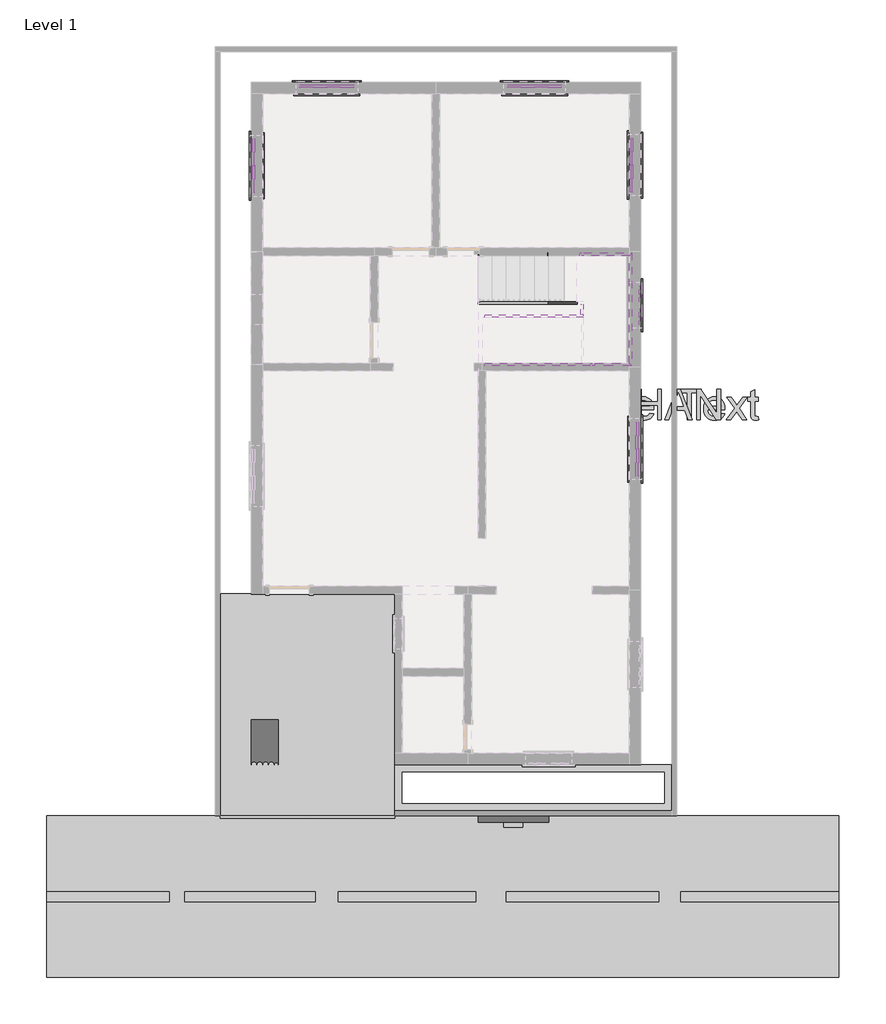
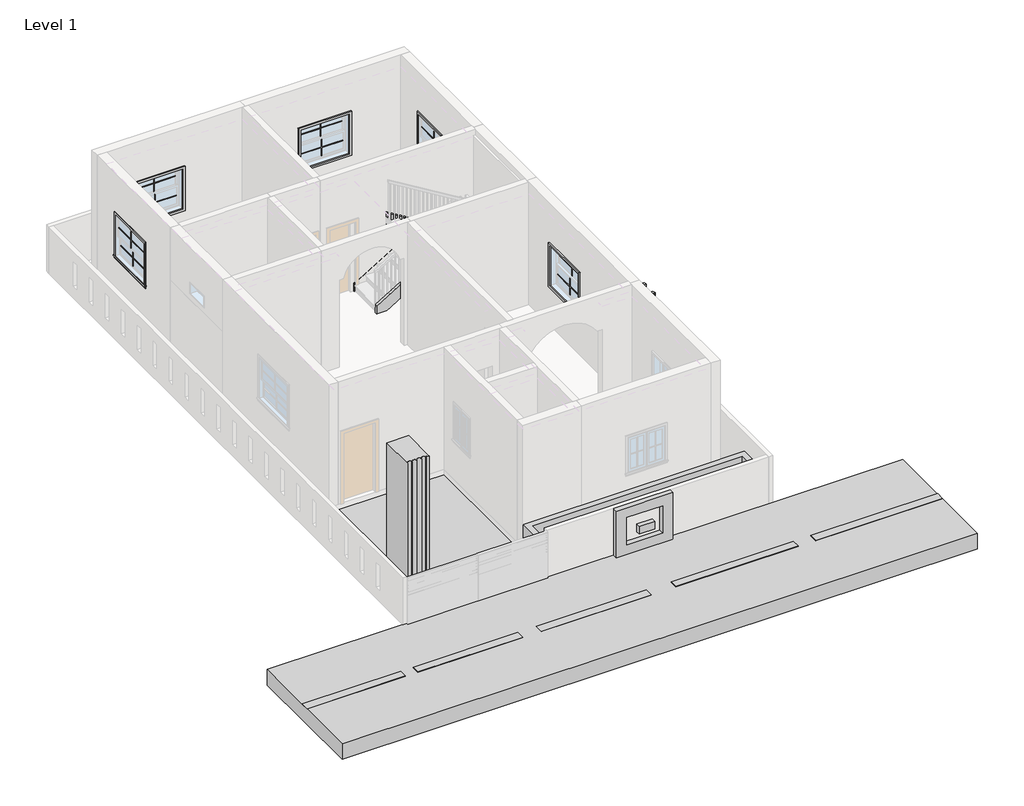
# One storey, part 3 of 3: 32 proxies, 8 members.
"""IFC4 building model written with IfcOpenShell, lengths in millimetres."""

from ifc_helpers import new_model, si_unit, frame, origin, origin_with_axes, place, context, project, spatial, polyline, outline, extrude, faceted_brep, transform, mapped, element, save
from components import generic_models_4629e616, design_design_48f371e7, generic_models_1_generic_models_1_2bf1bac3, generic_models_2_generic_models_2_314bea4d, muntin_pattern_2x2_muntin_pattern_2x2_8b3f23e7, muntin_pattern_2x2_muntin_pattern_2x2_5e52a1c6, muntin_pattern_2x2_muntin_pattern_2x2_d1c6e638, muntin_pattern_2x2_muntin_pattern_2x2_37b95fb2, trim_window_exterior_flat_with_sill_f44f30ad, trim_window_exterior_flat_with_sill_e2e7eb1d, trim_window_exterior_flat_with_sill_84e24481, trim_window_interior_flat_picture_frame_1dce1945, trim_window_interior_flat_picture_frame_a40cb921, trim_window_interior_flat_picture_frame_28d4e5dc

model = new_model("IFC4")

# Units and contexts
model_context = context("Model", 3, world=origin())
ifc_project = project(units=[si_unit("LENGTHUNIT", "METRE", prefix="MILLI")], contexts=[model_context])

# Site, building, storey
site = spatial("IfcSite", under=ifc_project)
building = spatial("IfcBuilding", under=site)
storey = spatial("IfcBuildingStorey", under=building, Name="Level 1", Elevation=0.0)

# Proxies
placement = place(None, origin())
generic_models_shape = generic_models_4629e616(model_context)
element("IfcBuildingElementProxy", 1, Name="Generic Models", at=placement, inside=storey, context=model_context, shape_type="MappedRepresentation", body=[
    mapped(generic_models_shape, transform((0.0, 0.0, 0.0), x_axis=(1.0, 0.0, 0.0), y_axis=(0.0, 1.0, 0.0), z_axis=(0.0, 0.0, 1.0))),
])
element("IfcBuildingElementProxy", 2, Name="24\" Arial", ObjectType="24\" Arial", at=placement, inside=storey, context=model_context, shape_type="SweptSolid", body=[
    extrude(outline(polyline([(66.6240518, 0.0), (66.6240518, 609.1341881), (197.1952963, 609.1341881), (322.1153934, 179.7957113), (347.3968417, 90.1209272), (374.6115771, 187.2314314), (497.1522439, 609.1341881), (628.1696315, 609.1341881), (628.1696315, 0.0), (552.027858, 0.0), (552.027858, 532.9924146), (399.000739, 0.0), (295.9416588, 0.0), (142.7658253, 532.9924146), (142.7658253, 0.0), (66.6240518, 0.0)])), origin_with_axes(), (0.0, 0.0, 1.0), 152.4),
    extrude(outline(polyline([(732.8645701, 223.6664597), (736.9821001, 281.6000137), (749.3346901, 331.5215793), (769.92234, 373.4311566), (798.7450499, 407.3287454), (827.7629475, 428.9945748), (859.7923117, 444.4701672), (894.8331425, 453.7555226), (932.88544, 456.8506411), (974.8926111, 453.0816605), (1012.8751986, 441.7747187), (1046.8332027, 422.9298156), (1076.7666233, 396.5469513), (1101.1976111, 363.5184122), (1118.6483166, 324.7364848), (1129.11874, 280.2011689), (1132.6088811, 229.9124646), (1131.0659692, 189.1554239), (1126.4372334, 152.9899404), (1118.7226738, 121.4160141), (1107.9222904, 94.4336449), (1094.1708556, 71.1273098), (1077.6031418, 50.5814858), (1058.2191491, 32.7961728), (1036.0188774, 17.771371), (1011.8667291, 5.8323929), (986.6271068, -2.6954485), (960.3000104, -7.8121534), (932.88544, -9.5177217), (890.264822, -5.7626831), (851.9290377, 5.5024329), (817.8780871, 24.277626), (788.1119702, 50.5628965), (763.9412327, 83.912101), (746.6764201, 123.8790964), (736.3175326, 170.4638826), (732.8645701, 223.6664597)]), holes=[polyline([(809.0063436, 223.8151741), (811.2091757, 186.882882), (817.8176719, 154.9046384), (828.8318323, 127.8804432), (844.2516568, 105.8102966), (863.0082606, 88.6663145), (884.0327591, 76.420613), (907.3251522, 69.0731921), (932.88544, 66.6240518), (958.3156026, 69.0871341), (981.5150492, 76.4763809), (1002.4837798, 88.7917923), (1021.2217944, 106.0333682), (1036.6416189, 128.3219391), (1047.6557793, 155.7783355), (1054.2642755, 188.4025573), (1056.4671075, 226.1946045), (1054.2503335, 261.9557707), (1047.6000114, 293.0974959), (1036.5161411, 319.6197799), (1020.9987228, 341.5226228), (1002.1909984, 358.6666049), (981.2362097, 370.9123064), (958.1343569, 378.2597273), (932.88544, 380.7088676), (907.3251522, 378.2690219), (884.0327591, 370.949485), (863.0082606, 358.7502568), (844.2516568, 341.6713372), (828.8318323, 319.6662531), (817.8176719, 292.6885313), (811.2091757, 260.7381716), (809.0063436, 223.8151741)])]), origin_with_axes(), (0.0, 0.0, 1.0), 152.4),
    extrude(outline(polyline([(1494.2823053, 0.0), (1494.2823053, 71.8290559), (1471.5011179, 36.2398407), (1443.9053018, 10.8189727), (1411.4948569, -4.4335481), (1374.2697833, -9.5177217), (1349.1370495, -7.677381), (1325.0453165, -2.1563588), (1301.9945843, 7.0453448), (1279.9848529, 19.9277298), (1259.7039264, 36.1050683), (1241.8396089, 55.1916322), (1226.3919004, 77.1874217), (1213.360801, 102.0924366), (1203.0158555, 129.4326498), (1195.6266087, 158.7340342), (1189.7152112, 223.2203165), (1195.1618762, 286.9072589), (1211.501871, 344.4225536), (1223.7522198, 370.0479039), (1238.7166065, 392.4944839), (1256.3950309, 411.7622935), (1276.7874932, 427.8513328), (1299.173658, 440.5385302), (1322.8331898, 449.600814), (1347.7660886, 455.0381843), (1373.9723545, 456.8506411), (1411.2253121, 451.6642264), (1444.165552, 436.1049821), (1472.0866809, 412.25491), (1494.2823053, 382.1960116), (1494.2823053, 609.1341881), (1570.4240788, 609.1341881), (1570.4240788, 0.0), (1494.2823053, 0.0)]), holes=[polyline([(1265.8569847, 223.5177453), (1268.0040489, 186.5947478), (1274.4452414, 154.6443882), (1285.1805623, 127.6666663), (1300.2100114, 105.6615822), (1318.1579808, 88.5826627), (1337.648862, 76.3834344), (1358.6826551, 69.0638975), (1381.2593602, 66.6240518), (1403.9429537, 68.9523617), (1424.8512691, 75.9372912), (1443.9843063, 87.5788404), (1461.3420654, 103.8770094), (1475.7534203, 124.9619231), (1486.0472453, 150.9637067), (1492.2235403, 181.8823602), (1494.2823053, 217.7178837), (1492.1863617, 257.0063696), (1485.8985309, 290.6994761), (1475.4188129, 318.7972034), (1460.7472078, 341.2995512), (1443.0083681, 358.5411271), (1423.3269465, 370.8565385), (1401.7029431, 378.2457853), (1378.1363578, 380.7088676), (1355.1135095, 378.3433791), (1334.0797164, 371.2469138), (1315.0349783, 359.4194716), (1297.9792954, 342.8610524), (1283.9257845, 321.2091651), (1273.8875624, 294.1013181), (1267.8646291, 261.5375115), (1265.8569847, 223.5177453)])]), origin_with_axes(), (0.0, 0.0, 1.0), 152.4),
    extrude(outline(polyline([(1997.8292684, 133.2481037), (2072.4838979, 123.730382), (2061.0375363, 93.8294926), (2045.5851806, 67.4791596), (2026.1268306, 44.679383), (2002.6624865, 25.4301626), (1975.433809, 10.1404632), (1944.6824592, -0.7807506), (1910.408437, -7.3334789), (1872.6117424, -9.5177217), (1825.367036, -5.7487411), (1783.2715658, 5.5582008), (1746.3253317, 24.4031038), (1714.5283337, 50.7859681), (1688.9587514, 83.9725162), (1670.6947639, 123.2284709), (1659.7363715, 168.553832), (1656.083574, 219.9485997), (1659.7735501, 273.0861142), (1670.8434783, 319.921856), (1689.2933588, 360.455825), (1715.1231914, 394.6880213), (1746.8365375, 421.8841675), (1782.9369584, 441.3099862), (1823.4244542, 452.9654774), (1868.2990248, 456.8506411), (1911.7282773, 452.974772), (1951.0028213, 441.3471648), (1986.1226566, 421.9678193), (2017.0877834, 394.8367357), (2042.3645843, 360.6788966), (2060.4194421, 320.2192848), (2071.2523568, 273.4579002), (2074.8633283, 220.3947429), (2074.4171851, 199.8721555), (1732.2253475, 199.8721555), (1736.635659, 169.4879443), (1745.4051613, 142.8773611), (1758.5338546, 120.0404059), (1776.0217387, 100.9770786), (1796.9021701, 85.9476294), (1820.2085052, 75.2123085), (1845.940744, 68.771116), (1874.0988864, 66.6240518), (1914.6235608, 70.6021621), (1948.753516, 82.5364928), (1976.4887518, 103.170616), (1997.8292684, 133.2481037)]), holes=[polyline([(1732.2253475, 276.013929), (1998.7215548, 276.013929), (1988.4230825, 316.2411746), (1979.565281, 332.060669), (1968.2351025, 345.0174112), (1947.4708542, 360.6324234), (1923.8438537, 371.7860035), (1897.354101, 378.4781516), (1868.001596, 380.7088676), (1841.2283564, 378.9289421), (1816.6765382, 373.5891656), (1794.3461414, 364.6895382), (1774.2371659, 352.2300597), (1757.3627287, 336.7869986), (1744.7359465, 318.9366231), (1736.3568195, 298.6789332), (1732.2253475, 276.013929)])]), origin_with_axes(), (0.0, 0.0, 1.0), 152.4),
    extrude(outline(polyline([(2151.0051019, 0.0), (2151.0051019, 609.1341881), (2227.1468754, 609.1341881), (2227.1468754, 0.0), (2151.0051019, 0.0)])), origin_with_axes(), (0.0, 0.0, 1.0), 152.4),
    extrude(outline(polyline([(2741.1038466, 0.0), (2741.1038466, 532.9924146), (2541.2316911, 532.9924146), (2541.2316911, 609.1341881), (3017.1177756, 609.1341881), (3017.1177756, 532.9924146), (2817.2456201, 532.9924146), (2817.2456201, 0.0), (2741.1038466, 0.0)])), origin_with_axes(), (0.0, 0.0, 1.0), 152.4),
    extrude(outline(polyline([(3406.4520785, 133.2481037), (3481.106708, 123.730382), (3469.6603464, 93.8294926), (3454.2079906, 67.4791596), (3434.7496407, 44.679383), (3411.2852965, 25.4301626), (3384.0566191, 10.1404632), (3353.3052693, -0.7807506), (3319.0312471, -7.3334789), (3281.2345525, -9.5177217), (3233.9898461, -5.7487411), (3191.8943759, 5.5582008), (3154.9481418, 24.4031038), (3123.1511438, 50.7859681), (3097.5815614, 83.9725162), (3079.317574, 123.2284709), (3068.3591815, 168.553832), (3064.7063841, 219.9485997), (3068.3963601, 273.0861142), (3079.4662884, 319.921856), (3097.9161688, 360.455825), (3123.7460014, 394.6880213), (3155.4593475, 421.8841675), (3191.5597685, 441.3099862), (3232.0472642, 452.9654774), (3276.9218349, 456.8506411), (3320.3510874, 452.974772), (3359.6256313, 441.3471648), (3394.7454667, 421.9678193), (3425.7105935, 394.8367357), (3450.9873944, 360.6788966), (3469.0422522, 320.2192848), (3479.8751668, 273.4579002), (3483.4861384, 220.3947429), (3483.0399952, 199.8721555), (3140.8481576, 199.8721555), (3145.258469, 169.4879443), (3154.0279714, 142.8773611), (3167.1566647, 120.0404059), (3184.6445488, 100.9770786), (3205.5249802, 85.9476294), (3228.8313153, 75.2123085), (3254.5635541, 68.771116), (3282.7216965, 66.6240518), (3323.2463709, 70.6021621), (3357.376326, 82.5364928), (3385.1115619, 103.170616), (3406.4520785, 133.2481037)]), holes=[polyline([(3140.8481576, 276.013929), (3407.3443649, 276.013929), (3397.0458926, 316.2411746), (3388.1880911, 332.060669), (3376.8579126, 345.0174112), (3356.0936643, 360.6324234), (3332.4666638, 371.7860035), (3305.976911, 378.4781516), (3276.6244061, 380.7088676), (3249.8511665, 378.9289421), (3225.2993483, 373.5891656), (3202.9689514, 364.6895382), (3182.859976, 352.2300597), (3165.9855387, 336.7869986), (3153.3587566, 318.9366231), (3144.9796295, 298.6789332), (3140.8481576, 276.013929)])]), origin_with_axes(), (0.0, 0.0, 1.0), 152.4),
    extrude(outline(polyline([(3512.0393035, 0.0), (3674.7328586, 225.0048893), (3521.5570252, 447.3329194), (3612.8676676, 447.3329194), (3686.7787251, 340.109836), (3721.4291806, 289.6956539), (3751.4694897, 331.0382575), (3835.6418409, 447.3329194), (3927.2499122, 447.3329194), (3766.3409299, 224.8561749), (3921.3013361, 0.0), (3829.8419793, 0.0), (3736.4493352, 135.3301053), (3719.4958934, 160.1654103), (3603.6473747, 0.0), (3512.0393035, 0.0)])), origin_with_axes(), (0.0, 0.0, 1.0), 152.4),
    extrude(outline(polyline([(4149.7266567, 63.5010494), (4159.2443784, -2.230716), (4129.0925335, -7.6959703), (4102.2867626, -9.5177217), (4065.7401985, -6.3575407), (4038.4882844, 3.1230024), (4019.2297695, 17.7341924), (4006.6634025, 36.2863139), (3999.7481829, 68.1483744), (3997.4431096, 122.6893812), (3997.4431096, 371.1911459), (3940.3367795, 371.1911459), (3940.3367795, 447.3329194), (3997.4431096, 447.3329194), (3997.4431096, 556.0431468), (4073.5848832, 600.8061817), (4073.5848832, 447.3329194), (4149.7266567, 447.3329194), (4149.7266567, 371.1911459), (4073.5848832, 371.1911459), (4073.5848832, 124.9200972), (4077.600172, 85.6594952), (4090.6126821, 71.7546987), (4101.5989585, 67.9067135), (4116.5633452, 66.6240518), (4149.7266567, 63.5010494)])), origin_with_axes(), (0.0, 0.0, 1.0), 152.4),
])
element("IfcBuildingElementProxy", 3, Name="24\" Arial", ObjectType="24\" Arial", at=placement, inside=storey, context=model_context, shape_type="SweptSolid", body=[
    extrude(outline(polyline([(66.6240518, 0.0), (66.6240518, 609.1341881), (475.8860845, 609.1341881), (475.8860845, 532.9924146), (142.7658253, 532.9924146), (142.7658253, 352.1557025), (428.297476, 352.1557025), (428.297476, 276.013929), (142.7658253, 276.013929), (142.7658253, 0.0), (66.6240518, 0.0)])), origin_with_axes(), (0.0, 0.0, 1.0), 152.4),
    extrude(outline(polyline([(-4.1640032, -732.1053287), (238.9840431, -122.9711405), (303.8235221, -122.9711405), (546.8228539, -732.1053287), (466.3683628, -732.1053287), (396.7700229, -541.7508949), (145.7401134, -541.7508949), (76.1417735, -732.1053287), (-4.1640032, -732.1053287)]), holes=[polyline([(173.6984208, -465.6091214), (368.9604299, -465.6091214), (313.9361014, -315.8537192), (271.2550682, -199.1129141), (233.3328958, -302.7668518), (173.6984208, -465.6091214)])]), origin_with_axes(), (0.0, 0.0, 1.0), 152.4),
    extrude(outline(polyline([(66.6240518, -1464.2106574), (66.6240518, -855.0764692), (329.1049703, -855.0764692), (399.6513645, -859.1847046), (450.9764222, -871.5094106), (470.7833216, -881.3059718), (488.48963, -894.262714), (504.0953475, -910.3796372), (517.6004741, -929.6567415), (528.4984513, -951.0576733), (536.2827208, -973.5460792), (540.9532824, -997.1219592), (542.5101363, -1021.7853132), (539.9308709, -1053.0711054), (532.1930747, -1081.7915742), (519.2967477, -1107.9467195), (501.2418899, -1131.5365414), (477.7961351, -1151.8081733), (448.7271169, -1168.0087484), (414.0348355, -1180.1382667), (373.7192907, -1188.1967284), (398.814846, -1204.5924911), (416.9951815, -1220.7651823), (448.1880272, -1257.7578896), (478.7116581, -1299.1376718), (580.2835943, -1464.2106574), (491.7985254, -1464.2106574), (412.5337495, -1337.9521306), (355.2787049, -1254.374637), (333.9939562, -1230.0040645), (315.0514594, -1214.8909634), (278.8395026, -1200.3913093), (234.6713254, -1197.71445), (142.7658253, -1197.71445), (142.7658253, -1464.2106574), (66.6240518, -1464.2106574)]), holes=[polyline([(142.7658253, -1121.5726765), (313.1925293, -1121.5726765), (362.1381567, -1118.877228), (400.116097, -1110.7908824), (428.7064406, -1096.7745501), (449.4892782, -1076.2891413), (462.1485917, -1051.5096042), (466.3683628, -1024.6108868), (464.356071, -1005.1385949), (458.3191958, -987.4694651), (448.2577371, -971.6034974), (434.1716949, -957.5406918), (415.7357564, -946.0246203), (392.624609, -937.798855), (364.8382526, -932.8633958), (332.3766871, -931.2182427), (142.7658253, -931.2182427), (142.7658253, -1121.5726765)])]), origin_with_axes(), (0.0, 0.0, 1.0), 152.4),
    extrude(outline(polyline([(66.6240518, -2196.315986), (66.6240518, -1587.1817979), (142.7658253, -1587.1817979), (142.7658253, -1834.6425618), (466.3683628, -1834.6425618), (466.3683628, -1587.1817979), (542.5101363, -1587.1817979), (542.5101363, -2196.315986), (466.3683628, -2196.315986), (466.3683628, -1910.7843353), (142.7658253, -1910.7843353), (142.7658253, -2196.315986), (66.6240518, -2196.315986)])), origin_with_axes(), (0.0, 0.0, 1.0), 152.4),
    extrude(outline(polyline([(-4.1640032, -2928.4213147), (238.9840431, -2319.2871266), (303.8235221, -2319.2871266), (546.8228539, -2928.4213147), (466.3683628, -2928.4213147), (396.7700229, -2738.0668809), (145.7401134, -2738.0668809), (76.1417735, -2928.4213147), (-4.1640032, -2928.4213147)]), holes=[polyline([(173.6984208, -2661.9251074), (368.9604299, -2661.9251074), (313.9361014, -2512.1697052), (271.2550682, -2395.4289001), (233.3328958, -2499.0828379), (173.6984208, -2661.9251074)])]), origin_with_axes(), (0.0, 0.0, 1.0), 152.4),
    extrude(outline(polyline([(66.6240518, -3660.5266434), (66.6240518, -3051.3924553), (148.1195438, -3051.3924553), (466.3683628, -3533.9706878), (466.3683628, -3051.3924553), (542.5101363, -3051.3924553), (542.5101363, -3660.5266434), (461.0146443, -3660.5266434), (142.7658253, -3177.7996964), (142.7658253, -3660.5266434), (66.6240518, -3660.5266434)])), origin_with_axes(), (0.0, 0.0, 1.0), 152.4),
])
element("IfcBuildingElementProxy", 4, Name="24\" Arial", ObjectType="24\" Arial", at=placement, inside=storey, context=model_context, shape_type="SweptSolid", body=[
    extrude(outline(polyline([(66.6240518, 0.0), (66.6240518, 609.1341881), (475.8860845, 609.1341881), (475.8860845, 532.9924146), (142.7658253, 532.9924146), (142.7658253, 352.1557025), (428.297476, 352.1557025), (428.297476, 276.013929), (142.7658253, 276.013929), (142.7658253, 0.0), (66.6240518, 0.0)])), origin_with_axes(), (0.0, 0.0, 1.0), 152.4),
    extrude(outline(polyline([(509.792968, 0.0), (752.9410143, 609.1341881), (817.7804933, 609.1341881), (1060.7798252, 0.0), (980.325334, 0.0), (910.7269942, 190.3544338), (659.6970846, 190.3544338), (590.0987448, 0.0), (509.792968, 0.0)]), holes=[polyline([(687.6553921, 266.4962073), (882.9174011, 266.4962073), (827.8930726, 416.2516095), (785.2120394, 532.9924146), (747.289867, 429.3384768), (687.6553921, 266.4962073)])]), origin_with_axes(), (0.0, 0.0, 1.0), 152.4),
    extrude(outline(polyline([(1142.1266028, 0.0), (1142.1266028, 609.1341881), (1404.6075212, 609.1341881), (1475.1539154, 605.0259528), (1526.4789732, 592.7012468), (1546.2858725, 582.9046856), (1563.9921809, 569.9479434), (1579.5978984, 553.8310201), (1593.103025, 534.5539158), (1604.0010022, 513.152984), (1611.7852717, 490.6645781), (1616.4558333, 467.0886982), (1618.0126872, 442.4253442), (1615.4334218, 411.139552), (1607.6956256, 382.4190832), (1594.7992986, 356.2639379), (1576.7444408, 332.6741159), (1553.298686, 312.4024841), (1524.2296679, 296.201909), (1489.5373864, 284.0723906), (1449.2218416, 276.013929), (1474.3173969, 259.6181662), (1492.4977325, 243.4454751), (1523.6905781, 206.4527677), (1554.214209, 165.0729856), (1655.7861452, 0.0), (1567.3010764, 0.0), (1488.0363004, 126.2585268), (1430.7812559, 209.8360204), (1409.4965072, 234.2065929), (1390.5540103, 249.3196939), (1354.3420536, 263.8193481), (1310.1738763, 266.4962073), (1218.2683763, 266.4962073), (1218.2683763, 0.0), (1142.1266028, 0.0)]), holes=[polyline([(1218.2683763, 342.6379808), (1388.6950803, 342.6379808), (1437.6407076, 345.3334294), (1475.6186479, 353.4197749), (1504.2089916, 367.4361073), (1524.9918292, 387.9215161), (1537.6511426, 412.7010532), (1541.8709137, 439.5997705), (1539.858622, 459.0720625), (1533.8217467, 476.7411923), (1523.760288, 492.60716), (1509.6742458, 506.6699656), (1491.2383074, 518.186037), (1468.1271599, 526.4118024), (1440.3408035, 531.3472616), (1407.8792381, 532.9924146), (1218.2683763, 532.9924146), (1218.2683763, 342.6379808)])]), origin_with_axes(), (0.0, 0.0, 1.0), 152.4),
    extrude(outline(polyline([(1751.2607909, 0.0), (1751.2607909, 609.1341881), (1827.4025644, 609.1341881), (1827.4025644, 361.6734242), (2151.0051019, 361.6734242), (2151.0051019, 609.1341881), (2227.1468754, 609.1341881), (2227.1468754, 0.0), (2151.0051019, 0.0), (2151.0051019, 285.5316507), (1827.4025644, 285.5316507), (1827.4025644, 0.0), (1751.2607909, 0.0)])), origin_with_axes(), (0.0, 0.0, 1.0), 152.4),
    extrude(outline(polyline([(2289.606924, 0.0), (2532.7549703, 609.1341881), (2597.5944493, 609.1341881), (2840.5937812, 0.0), (2760.13929, 0.0), (2690.5409501, 190.3544338), (2439.5110406, 190.3544338), (2369.9127007, 0.0), (2289.606924, 0.0)]), holes=[polyline([(2467.469348, 266.4962073), (2662.7313571, 266.4962073), (2607.7070286, 416.2516095), (2565.0259954, 532.9924146), (2527.103823, 429.3384768), (2467.469348, 266.4962073)])]), origin_with_axes(), (0.0, 0.0, 1.0), 152.4),
    extrude(outline(polyline([(2921.9405587, 0.0), (2921.9405587, 609.1341881), (3003.4360507, 609.1341881), (3321.6848697, 126.5559556), (3321.6848697, 609.1341881), (3397.8266432, 609.1341881), (3397.8266432, 0.0), (3316.3311512, 0.0), (2998.0823322, 482.7269469), (2998.0823322, 0.0), (2921.9405587, 0.0)])), origin_with_axes(), (0.0, 0.0, 1.0), 152.4),
])
element("IfcBuildingElementProxy", 5, Name="24\" Arial", ObjectType="24\" Arial", at=placement, inside=storey, context=model_context, shape_type="SweptSolid", body=[
    extrude(outline(polyline([(66.6240518, 0.0), (66.6240518, 609.1341881), (475.8860845, 609.1341881), (475.8860845, 532.9924146), (142.7658253, 532.9924146), (142.7658253, 352.1557025), (428.297476, 352.1557025), (428.297476, 276.013929), (142.7658253, 276.013929), (142.7658253, 0.0), (66.6240518, 0.0)])), origin_with_axes(), (0.0, 0.0, 1.0), 152.4),
    extrude(outline(polyline([(509.792968, 0.0), (752.9410143, 609.1341881), (817.7804933, 609.1341881), (1060.7798252, 0.0), (980.325334, 0.0), (910.7269942, 190.3544338), (659.6970846, 190.3544338), (590.0987448, 0.0), (509.792968, 0.0)]), holes=[polyline([(687.6553921, 266.4962073), (882.9174011, 266.4962073), (827.8930726, 416.2516095), (785.2120394, 532.9924146), (747.289867, 429.3384768), (687.6553921, 266.4962073)])]), origin_with_axes(), (0.0, 0.0, 1.0), 152.4),
    extrude(outline(polyline([(1142.1266028, 0.0), (1142.1266028, 609.1341881), (1404.6075212, 609.1341881), (1475.1539154, 605.0259528), (1526.4789732, 592.7012468), (1546.2858725, 582.9046856), (1563.9921809, 569.9479434), (1579.5978984, 553.8310201), (1593.103025, 534.5539158), (1604.0010022, 513.152984), (1611.7852717, 490.6645781), (1616.4558333, 467.0886982), (1618.0126872, 442.4253442), (1615.4334218, 411.139552), (1607.6956256, 382.4190832), (1594.7992986, 356.2639379), (1576.7444408, 332.6741159), (1553.298686, 312.4024841), (1524.2296679, 296.201909), (1489.5373864, 284.0723906), (1449.2218416, 276.013929), (1474.3173969, 259.6181662), (1492.4977325, 243.4454751), (1523.6905781, 206.4527677), (1554.214209, 165.0729856), (1655.7861452, 0.0), (1567.3010764, 0.0), (1488.0363004, 126.2585268), (1430.7812559, 209.8360204), (1409.4965072, 234.2065929), (1390.5540103, 249.3196939), (1354.3420536, 263.8193481), (1310.1738763, 266.4962073), (1218.2683763, 266.4962073), (1218.2683763, 0.0), (1142.1266028, 0.0)]), holes=[polyline([(1218.2683763, 342.6379808), (1388.6950803, 342.6379808), (1437.6407076, 345.3334294), (1475.6186479, 353.4197749), (1504.2089916, 367.4361073), (1524.9918292, 387.9215161), (1537.6511426, 412.7010532), (1541.8709137, 439.5997705), (1539.858622, 459.0720625), (1533.8217467, 476.7411923), (1523.760288, 492.60716), (1509.6742458, 506.6699656), (1491.2383074, 518.186037), (1468.1271599, 526.4118024), (1440.3408035, 531.3472616), (1407.8792381, 532.9924146), (1218.2683763, 532.9924146), (1218.2683763, 342.6379808)])]), origin_with_axes(), (0.0, 0.0, 1.0), 152.4),
    extrude(outline(polyline([(1751.2607909, 0.0), (1751.2607909, 609.1341881), (1827.4025644, 609.1341881), (1827.4025644, 361.6734242), (2151.0051019, 361.6734242), (2151.0051019, 609.1341881), (2227.1468754, 609.1341881), (2227.1468754, 0.0), (2151.0051019, 0.0), (2151.0051019, 285.5316507), (1827.4025644, 285.5316507), (1827.4025644, 0.0), (1751.2607909, 0.0)])), origin_with_axes(), (0.0, 0.0, 1.0), 152.4),
    extrude(outline(polyline([(2289.606924, 0.0), (2532.7549703, 609.1341881), (2597.5944493, 609.1341881), (2840.5937812, 0.0), (2760.13929, 0.0), (2690.5409501, 190.3544338), (2439.5110406, 190.3544338), (2369.9127007, 0.0), (2289.606924, 0.0)]), holes=[polyline([(2467.469348, 266.4962073), (2662.7313571, 266.4962073), (2607.7070286, 416.2516095), (2565.0259954, 532.9924146), (2527.103823, 429.3384768), (2467.469348, 266.4962073)])]), origin_with_axes(), (0.0, 0.0, 1.0), 152.4),
    extrude(outline(polyline([(2921.9405587, 0.0), (2921.9405587, 609.1341881), (3003.4360507, 609.1341881), (3321.6848697, 126.5559556), (3321.6848697, 609.1341881), (3397.8266432, 609.1341881), (3397.8266432, 0.0), (3316.3311512, 0.0), (2998.0823322, 482.7269469), (2998.0823322, 0.0), (2921.9405587, 0.0)])), origin_with_axes(), (0.0, 0.0, 1.0), 152.4),
])
design_design_shape = design_design_48f371e7(model_context)
element("IfcBuildingElementProxy", 6, Name="DESIGN : DESIGN", ObjectType="DESIGN : DESIGN", at=placement, inside=storey, context=model_context, shape_type="MappedRepresentation", body=[
    mapped(design_design_shape, transform((0.0, 0.0, 0.0), x_axis=(1.0, 0.0, 0.0), y_axis=(0.0, 1.0, 0.0), z_axis=(0.0, 0.0, 1.0))),
])
generic_models_1_generic_models_1_shape = generic_models_1_generic_models_1_2bf1bac3(model_context)
element("IfcBuildingElementProxy", 7, Name="Generic Models 1 : Generic Models 1", ObjectType="Generic Models 1 : Generic Models 1", at=placement, inside=storey, context=model_context, shape_type="MappedRepresentation", body=[
    mapped(generic_models_1_generic_models_1_shape, transform((0.0, 0.0, 0.0), x_axis=(1.0, 0.0, 0.0), y_axis=(0.0, 1.0, 0.0), z_axis=(0.0, 0.0, 1.0))),
])
generic_models_2_generic_models_2_shape = generic_models_2_generic_models_2_314bea4d(model_context)
element("IfcBuildingElementProxy", 8, Name="Generic Models 2 : Generic Models 2", ObjectType="Generic Models 2 : Generic Models 2", at=placement, inside=storey, context=model_context, shape_type="MappedRepresentation", body=[
    mapped(generic_models_2_generic_models_2_shape, transform((0.0, 0.0, 0.0), x_axis=(1.0, 0.0, 0.0), y_axis=(0.0, 1.0, 0.0), z_axis=(0.0, 0.0, 1.0))),
])
muntin_pattern_2x2_muntin_pattern_2x2_shape = muntin_pattern_2x2_muntin_pattern_2x2_8b3f23e7(model_context)
element("IfcBuildingElementProxy", 9, Name="Muntin Pattern_2x2 : Muntin Pattern_2x2", ObjectType="Muntin Pattern_2x2 : Muntin Pattern_2x2", at=placement, inside=storey, context=model_context, shape_type="MappedRepresentation", body=[
    mapped(muntin_pattern_2x2_muntin_pattern_2x2_shape, transform((-5865.439062, 5032.1857363, 1774.825), x_axis=(0.0, 1.0, 0.0), y_axis=(-1.0, 0.0, 0.0), z_axis=(0.0, 0.0, 1.0))),
])
element("IfcBuildingElementProxy", 10, Name="Muntin Pattern_2x2 : Muntin Pattern_2x2", ObjectType="Muntin Pattern_2x2 : Muntin Pattern_2x2", at=placement, inside=storey, context=model_context, shape_type="MappedRepresentation", body=[
    mapped(muntin_pattern_2x2_muntin_pattern_2x2_shape, transform((-5820.989062, 5032.1857363, 1295.4), x_axis=(0.0, 1.0, 0.0), y_axis=(-1.0, 0.0, 0.0), z_axis=(0.0, 0.0, 1.0))),
])
element("IfcBuildingElementProxy", 11, Name="Muntin Pattern_2x2 : Muntin Pattern_2x2", ObjectType="Muntin Pattern_2x2 : Muntin Pattern_2x2", at=placement, inside=storey, context=model_context, shape_type="MappedRepresentation", body=[
    mapped(muntin_pattern_2x2_muntin_pattern_2x2_shape, transform((1786.310938, -581.2142637, 1774.825), x_axis=(0.0, -1.0, 0.0), y_axis=(1.0, 0.0, 0.0), z_axis=(0.0, 0.0, 1.0))),
])
element("IfcBuildingElementProxy", 12, Name="Muntin Pattern_2x2 : Muntin Pattern_2x2", ObjectType="Muntin Pattern_2x2 : Muntin Pattern_2x2", at=placement, inside=storey, context=model_context, shape_type="MappedRepresentation", body=[
    mapped(muntin_pattern_2x2_muntin_pattern_2x2_shape, transform((1741.860938, -581.2142637, 1295.4), x_axis=(0.0, -1.0, 0.0), y_axis=(1.0, 0.0, 0.0), z_axis=(0.0, 0.0, 1.0))),
])
muntin_pattern_2x2_muntin_pattern_2x2_2_shape = muntin_pattern_2x2_muntin_pattern_2x2_5e52a1c6(model_context)
element("IfcBuildingElementProxy", 13, Name="Muntin Pattern_2x2 : Muntin Pattern_2x2", ObjectType="Muntin Pattern_2x2 : Muntin Pattern_2x2", at=placement, inside=storey, context=model_context, shape_type="MappedRepresentation", body=[
    mapped(muntin_pattern_2x2_muntin_pattern_2x2_2_shape, transform((-4401.764062, 6648.2607363, 1774.825), x_axis=(-1.0, 0.0, 0.0), y_axis=(0.0, -1.0, 0.0), z_axis=(0.0, 0.0, 1.0))),
])
element("IfcBuildingElementProxy", 14, Name="Muntin Pattern_2x2 : Muntin Pattern_2x2", ObjectType="Muntin Pattern_2x2 : Muntin Pattern_2x2", at=placement, inside=storey, context=model_context, shape_type="MappedRepresentation", body=[
    mapped(muntin_pattern_2x2_muntin_pattern_2x2_2_shape, transform((-4401.764062, 6603.8107363, 1295.4), x_axis=(-1.0, 0.0, 0.0), y_axis=(0.0, -1.0, 0.0), z_axis=(0.0, 0.0, 1.0))),
])
element("IfcBuildingElementProxy", 15, Name="Muntin Pattern_2x2 : Muntin Pattern_2x2", ObjectType="Muntin Pattern_2x2 : Muntin Pattern_2x2", at=placement, inside=storey, context=model_context, shape_type="MappedRepresentation", body=[
    mapped(muntin_pattern_2x2_muntin_pattern_2x2_2_shape, transform((-286.964062, 6648.2607363, 1774.825), x_axis=(-1.0, 0.0, 0.0), y_axis=(0.0, -1.0, 0.0), z_axis=(0.0, 0.0, 1.0))),
])
element("IfcBuildingElementProxy", 16, Name="Muntin Pattern_2x2 : Muntin Pattern_2x2", ObjectType="Muntin Pattern_2x2 : Muntin Pattern_2x2", at=placement, inside=storey, context=model_context, shape_type="MappedRepresentation", body=[
    mapped(muntin_pattern_2x2_muntin_pattern_2x2_2_shape, transform((-286.964062, 6603.8107363, 1295.4), x_axis=(-1.0, 0.0, 0.0), y_axis=(0.0, -1.0, 0.0), z_axis=(0.0, 0.0, 1.0))),
])
element("IfcBuildingElementProxy", 17, Name="Muntin Pattern_2x2 : Muntin Pattern_2x2", ObjectType="Muntin Pattern_2x2 : Muntin Pattern_2x2", at=placement, inside=storey, context=model_context, shape_type="MappedRepresentation", body=[
    mapped(muntin_pattern_2x2_muntin_pattern_2x2_2_shape, transform((1627.560938, 5044.8857363, 1774.825), x_axis=(0.0, -1.0, 0.0), y_axis=(1.0, 0.0, 0.0), z_axis=(0.0, 0.0, 1.0))),
])
element("IfcBuildingElementProxy", 18, Name="Muntin Pattern_2x2 : Muntin Pattern_2x2", ObjectType="Muntin Pattern_2x2 : Muntin Pattern_2x2", at=placement, inside=storey, context=model_context, shape_type="MappedRepresentation", body=[
    mapped(muntin_pattern_2x2_muntin_pattern_2x2_2_shape, transform((1672.010938, 5044.8857363, 1295.4), x_axis=(0.0, -1.0, 0.0), y_axis=(1.0, 0.0, 0.0), z_axis=(0.0, 0.0, 1.0))),
])
muntin_pattern_2x2_muntin_pattern_2x2_3_shape = muntin_pattern_2x2_muntin_pattern_2x2_d1c6e638(model_context)
element("IfcBuildingElementProxy", 19, Name="Muntin Pattern_2x2 : Muntin Pattern_2x2", ObjectType="Muntin Pattern_2x2 : Muntin Pattern_2x2", at=placement, inside=storey, context=model_context, shape_type="MappedRepresentation", body=[
    mapped(muntin_pattern_2x2_muntin_pattern_2x2_3_shape, transform((1811.710938, 2496.9482363, 1289.05), x_axis=(0.0, -1.0, 0.0), y_axis=(1.0, 0.0, 0.0), z_axis=(0.0, 0.0, 1.0))),
])
muntin_pattern_2x2_muntin_pattern_2x2_4_shape = muntin_pattern_2x2_muntin_pattern_2x2_37b95fb2(model_context)
element("IfcBuildingElementProxy", 20, Name="Muntin Pattern_2x2 : Muntin Pattern_2x2", ObjectType="Muntin Pattern_2x2 : Muntin Pattern_2x2", at=placement, inside=storey, context=model_context, shape_type="MappedRepresentation", body=[
    mapped(muntin_pattern_2x2_muntin_pattern_2x2_4_shape, transform((1811.710938, 2042.9232363, 1289.05), x_axis=(0.0, 1.0, 0.0), y_axis=(-1.0, 0.0, 0.0), z_axis=(0.0, 0.0, 1.0))),
])
trim_window_exterior_flat_with_sill_shape = trim_window_exterior_flat_with_sill_f44f30ad(model_context)
element("IfcBuildingElementProxy", 21, Name="Trim-Window-Exterior-Flat : with Sill", ObjectType="Trim-Window-Exterior-Flat : with Sill", at=placement, inside=storey, context=model_context, shape_type="MappedRepresentation", body=[
    mapped(trim_window_exterior_flat_with_sill_shape, transform((-5900.364062, 5032.1857363, 2286.0), x_axis=(0.0, -1.0, 0.0), y_axis=(0.0, 0.0, 1.0), z_axis=(-1.0, 0.0, 0.0))),
])
element("IfcBuildingElementProxy", 22, Name="Trim-Window-Exterior-Flat : with Sill", ObjectType="Trim-Window-Exterior-Flat : with Sill", at=placement, inside=storey, context=model_context, shape_type="MappedRepresentation", body=[
    mapped(trim_window_exterior_flat_with_sill_shape, transform((1821.235938, -581.2142637, 2286.0), x_axis=(0.0, 1.0, 0.0), y_axis=(0.0, 0.0, 1.0), z_axis=(1.0, 0.0, 0.0))),
])
trim_window_exterior_flat_with_sill_2_shape = trim_window_exterior_flat_with_sill_e2e7eb1d(model_context)
element("IfcBuildingElementProxy", 23, Name="Trim-Window-Exterior-Flat : with Sill", ObjectType="Trim-Window-Exterior-Flat : with Sill", at=placement, inside=storey, context=model_context, shape_type="MappedRepresentation", body=[
    mapped(trim_window_exterior_flat_with_sill_2_shape, transform((-4401.764062, 6683.1857363, 2286.0), x_axis=(1.0, 0.0, 0.0), y_axis=(0.0, 0.0, -1.0), z_axis=(0.0, 1.0, 0.0))),
])
element("IfcBuildingElementProxy", 24, Name="Trim-Window-Exterior-Flat : with Sill", ObjectType="Trim-Window-Exterior-Flat : with Sill", at=placement, inside=storey, context=model_context, shape_type="MappedRepresentation", body=[
    mapped(trim_window_exterior_flat_with_sill_2_shape, transform((-286.964062, 6683.1857363, 2286.0), x_axis=(1.0, 0.0, 0.0), y_axis=(0.0, 0.0, -1.0), z_axis=(0.0, 1.0, 0.0))),
])
element("IfcBuildingElementProxy", 25, Name="Trim-Window-Exterior-Flat : with Sill", ObjectType="Trim-Window-Exterior-Flat : with Sill", at=placement, inside=storey, context=model_context, shape_type="MappedRepresentation", body=[
    mapped(trim_window_exterior_flat_with_sill_2_shape, transform((1592.635938, 5044.8857363, 2286.0), x_axis=(0.0, 1.0, 0.0), y_axis=(0.0, 0.0, -1.0), z_axis=(-1.0, 0.0, 0.0))),
])
trim_window_exterior_flat_with_sill_3_shape = trim_window_exterior_flat_with_sill_84e24481(model_context)
element("IfcBuildingElementProxy", 26, Name="Trim-Window-Exterior-Flat : with Sill", ObjectType="Trim-Window-Exterior-Flat : with Sill", at=placement, inside=storey, context=model_context, shape_type="MappedRepresentation", body=[
    mapped(trim_window_exterior_flat_with_sill_3_shape, transform((1821.235938, 2269.9357363, 2133.6), x_axis=(0.0, 1.0, 0.0), y_axis=(0.0, 0.0, 1.0), z_axis=(1.0, 0.0, 0.0))),
])
trim_window_interior_flat_picture_frame_shape = trim_window_interior_flat_picture_frame_1dce1945(model_context)
element("IfcBuildingElementProxy", 27, Name="Trim-Window-Interior-Flat : Picture Frame", ObjectType="Trim-Window-Interior-Flat : Picture Frame", at=placement, inside=storey, context=model_context, shape_type="MappedRepresentation", body=[
    mapped(trim_window_interior_flat_picture_frame_shape, transform((-5671.764062, 5032.1857363, 2286.0), x_axis=(0.0, 1.0, 0.0), y_axis=(0.0, 0.0, 1.0), z_axis=(1.0, 0.0, 0.0))),
])
element("IfcBuildingElementProxy", 28, Name="Trim-Window-Interior-Flat : Picture Frame", ObjectType="Trim-Window-Interior-Flat : Picture Frame", at=placement, inside=storey, context=model_context, shape_type="MappedRepresentation", body=[
    mapped(trim_window_interior_flat_picture_frame_shape, transform((1592.635938, -581.2142637, 2286.0), x_axis=(0.0, -1.0, 0.0), y_axis=(0.0, 0.0, 1.0), z_axis=(-1.0, 0.0, 0.0))),
])
trim_window_interior_flat_picture_frame_2_shape = trim_window_interior_flat_picture_frame_a40cb921(model_context)
element("IfcBuildingElementProxy", 29, Name="Trim-Window-Interior-Flat : Picture Frame", ObjectType="Trim-Window-Interior-Flat : Picture Frame", at=placement, inside=storey, context=model_context, shape_type="MappedRepresentation", body=[
    mapped(trim_window_interior_flat_picture_frame_2_shape, transform((-4401.764062, 6454.5857363, 2286.0), x_axis=(-1.0, 0.0, 0.0), y_axis=(0.0, 0.0, -1.0), z_axis=(0.0, -1.0, 0.0))),
])
element("IfcBuildingElementProxy", 30, Name="Trim-Window-Interior-Flat : Picture Frame", ObjectType="Trim-Window-Interior-Flat : Picture Frame", at=placement, inside=storey, context=model_context, shape_type="MappedRepresentation", body=[
    mapped(trim_window_interior_flat_picture_frame_2_shape, transform((-286.964062, 6454.5857363, 2286.0), x_axis=(-1.0, 0.0, 0.0), y_axis=(0.0, 0.0, -1.0), z_axis=(0.0, -1.0, 0.0))),
])
element("IfcBuildingElementProxy", 31, Name="Trim-Window-Interior-Flat : Picture Frame", ObjectType="Trim-Window-Interior-Flat : Picture Frame", at=placement, inside=storey, context=model_context, shape_type="MappedRepresentation", body=[
    mapped(trim_window_interior_flat_picture_frame_2_shape, transform((1821.235938, 5044.8857363, 2286.0), x_axis=(0.0, -1.0, 0.0), y_axis=(0.0, 0.0, -1.0), z_axis=(1.0, 0.0, 0.0))),
])
trim_window_interior_flat_picture_frame_3_shape = trim_window_interior_flat_picture_frame_28d4e5dc(model_context)
element("IfcBuildingElementProxy", 32, Name="Trim-Window-Interior-Flat : Picture Frame", ObjectType="Trim-Window-Interior-Flat : Picture Frame", at=placement, inside=storey, context=model_context, shape_type="MappedRepresentation", body=[
    mapped(trim_window_interior_flat_picture_frame_3_shape, transform((1592.635938, 2269.9357363, 2133.6), x_axis=(0.0, -1.0, 0.0), y_axis=(0.0, 0.0, 1.0), z_axis=(-1.0, 0.0, 0.0))),
])

# Members
element("IfcMember", 33, ObjectType="Stringer - 2\" Width", at=placement, inside=storey, context=model_context, shape_type="SweptSolid", body=[
    extrude(outline(polyline([(364.514512, -1404.564062), (152.4, -1404.564062), (152.4, -1166.4785503), (1278.4666667, 691.5314497), (1583.2666667, 606.3769932), (364.514512, -1404.564062)])), frame((0.0, 3254.1857363, 0.0), z_axis=(0.0, 1.0, 0.0), x_axis=(0.0, 0.0, 1.0)), (0.0, 0.0, 1.0), 50.8),
])
element("IfcMember", 34, ObjectType="Stringer - 2\" Width", at=placement, inside=storey, context=model_context, shape_type="SweptSolid", body=[
    extrude(outline(polyline([(364.514512, -1404.564062), (152.4, -1404.564062), (152.4, -1166.4785503), (1270.4087807, 678.235938), (1583.2666667, 678.235938), (1583.2666667, 606.3769932), (364.514512, -1404.564062)])), frame((0.0, 2288.9857363, 0.0), z_axis=(0.0, 1.0, 0.0), x_axis=(0.0, 0.0, 1.0)), (0.0, 0.0, 1.0), 50.8),
])
element("IfcMember", 35, ObjectType="Stringer - 2\" Width", at=placement, inside=storey, context=model_context, shape_type="SweptSolid", body=[
    extrude(outline(polyline([(1278.4666667, 817.3404262), (1583.2666667, 902.4948827), (2904.514512, -1277.564062), (2548.1057504, -1277.564062), (1278.4666667, 817.3404262)])), frame((0.0, 1069.7857363, 0.0), z_axis=(0.0, 1.0, 0.0), x_axis=(0.0, 0.0, 1.0)), (0.0, 0.0, 1.0), 50.8),
])
element("IfcMember", 36, ObjectType="Stringer - 2\" Width", at=placement, inside=storey, context=model_context, shape_type="SweptSolid", body=[
    extrude(outline(polyline([(1362.7724171, 678.235938), (1719.1811786, 678.235938), (2904.514512, -1277.564062), (2548.1057504, -1277.564062), (1362.7724171, 678.235938)])), frame((0.0, 2034.9857363, 0.0), z_axis=(0.0, 1.0, 0.0), x_axis=(0.0, 0.0, 1.0)), (0.0, 0.0, 1.0), 50.8),
])
element("IfcMember", 37, ObjectType="Stringer - 2\" Width", at=placement, inside=storey, context=model_context, shape_type="Brep", body=[
    faceted_brep([(902.4948827, 1120.5857363, 1583.2666667), (902.4948827, 1069.7857363, 1583.2666667), (1643.435938, 1069.7857363, 1583.2666667), (1592.635938, 1120.5857363, 1583.2666667), (817.3404262, 1120.5857363, 1278.4666667), (1592.635938, 1120.5857363, 1278.4666667), (817.3404262, 1069.7857363, 1278.4666667), (1643.435938, 1069.7857363, 1278.4666667)], [[[0, 1, 2, 3]], [[4, 0, 3, 5]], [[6, 4, 5, 7]], [[1, 6, 7, 2]], [[1, 0, 4, 6]], [[2, 7, 5, 3]]]),
])
element("IfcMember", 38, ObjectType="Stringer - 2\" Width", at=placement, inside=storey, context=model_context, shape_type="SweptSolid", body=[
    extrude(outline(polyline([(1643.435938, 1069.7857363), (1592.635938, 1120.5857363), (1592.635938, 3254.1857363), (1643.435938, 3304.9857363), (1643.435938, 1069.7857363)])), frame((0.0, 0.0, 1278.4666667), z_axis=(0.0, 0.0, 1.0), x_axis=(1.0, 0.0, 0.0)), (0.0, 0.0, 1.0), 304.8),
])
element("IfcMember", 39, ObjectType="Stringer - 2\" Width", at=placement, inside=storey, context=model_context, shape_type="Brep", body=[
    faceted_brep([(1592.635938, 3254.1857363, 1583.2666667), (1643.435938, 3304.9857363, 1583.2666667), (606.3769932, 3304.9857363, 1583.2666667), (606.3769932, 3254.1857363, 1583.2666667), (1592.635938, 3254.1857363, 1278.4666667), (691.5314497, 3254.1857363, 1278.4666667), (1643.435938, 3304.9857363, 1278.4666667), (691.5314497, 3304.9857363, 1278.4666667)], [[[0, 1, 2, 3]], [[4, 0, 3, 5]], [[6, 4, 5, 7]], [[1, 6, 7, 2]], [[1, 0, 4, 6]], [[2, 7, 5, 3]]]),
])
element("IfcMember", 40, ObjectType="Stringer - 2\" Width", at=placement, inside=storey, context=model_context, shape_type="SweptSolid", body=[
    extrude(outline(polyline([(627.435938, 2288.9857363), (678.235938, 2288.9857363), (678.235938, 2085.7857363), (627.435938, 2085.7857363), (627.435938, 2288.9857363)])), frame((0.0, 0.0, 1278.4666667), z_axis=(0.0, 0.0, 1.0), x_axis=(1.0, 0.0, 0.0)), (0.0, 0.0, 1.0), 304.8),
])

save(model, "model.ifc")

# Revit data of these elements
# Type "Muntin Pattern_2x2 : Muntin Pattern_2x2"
#   Width [instance default] = 4' - 0"
#   Thickness = 0' - 0 1/2"
#   Height [instance default] = 4' - 0"
#   Distance = 0' - 0 3/4"
#   Interior Material [instance default] = none
#   Exterior Material [instance default] = none
#   Default Elevation = 0
# Type "Trim-Window-Exterior-Flat : with Sill"
#   Trim Width = 0' - 2 1/4"
#   Trim Thickness_Picture Frame = 0' - 1 1/4"
#   Trim Thickness_with Sill = 0' - 0 3/4"
#   Sill Thickness = 0' - 1 1/4"
#   Opening Width [instance default] = 2' - 0"
#   Opening Height [instance default] = 3' - 0"
#   Default Elevation = 4' - 0"
#   Sill = yes
#   Picture Frame = no
#   Trim Material [instance default] = none
# Type "Trim-Window-Interior-Flat : Picture Frame"
#   Trim Thickness_Picture Frame = 0' - 1 1/4"
#   Trim Width = 0' - 2 1/4"
#   Trim Thickness_with Sill = 0' - 0 3/4"
#   Sill Thickness = 0' - 1 1/4"
#   Opening Width [instance default] = 2' - 0"
#   Opening Height [instance default] = 3' - 0"
#   Default Elevation = 4' - 0"
#   Sill = no
#   Picture Frame = yes
#   Trim Material [instance default] = none
# Element 1 (IfcBuildingElementProxy)
#   Phase Created = New Construction
# Elements 2, 3, 4, 5 (IfcBuildingElementProxy, "24\" Arial")
#   Phase Created = New Construction
# Element 6 (IfcBuildingElementProxy, "DESIGN : DESIGN")
#   Phase Created = New Construction
#   Materials on its faces: "DINING ROOM WALL"
# Element 7 (IfcBuildingElementProxy, "Generic Models 1 : Generic Models 1")
#   Phase Created = New Construction
#   Materials on its faces: "FLOOR TILES", "BURGUNDY COLOUR", "LIVING ROOM WALL"
# Element 8 (IfcBuildingElementProxy, "Generic Models 2 : Generic Models 2")
#   Phase Created = New Construction
#   Materials on its faces: "ROAD"
# Elements 9, 10, 11, 12, 13, 14, 15, 16, 17, 18 (IfcBuildingElementProxy, "Muntin Pattern_2x2 : Muntin Pattern_2x2")
#   Width = 3' - 6"
#   Height = 1' - 5 1/8"
#   Interior Material = Wood - Stained
#   Exterior Material = Clad - White
#   Phase Created = New Construction
#   Materials on its faces: "Clad - White", "Wood - Stained"
# Elements 19, 20 (IfcBuildingElementProxy, "Muntin Pattern_2x2 : Muntin Pattern_2x2")
#   Width = 1' - 0 5/8"
#   Height = 2' - 6 1/2"
#   Interior Material = Wood - Stained
#   Exterior Material = Clad - White
#   Phase Created = New Construction
#   Materials on its faces: "Clad - White", "Wood - Stained"
# Elements 21, 22, 23, 24, 25 (IfcBuildingElementProxy, "Trim-Window-Exterior-Flat : with Sill")
#   Opening Width = 4' - 0"
#   Opening Height = 3' - 6"
#   Trim Material = Clad - White
#   Phase Created = New Construction
#   Materials on its faces: "Clad - White"
# Element 26 (IfcBuildingElementProxy, "Trim-Window-Exterior-Flat : with Sill")
#   Opening Width = 3' - 0"
#   Opening Height = 3' - 0"
#   Trim Material = Clad - White
#   Phase Created = New Construction
#   Materials on its faces: "Clad - White"
# Elements 27, 28, 29, 30, 31 (IfcBuildingElementProxy, "Trim-Window-Interior-Flat : Picture Frame")
#   Opening Width = 4' - 0"
#   Opening Height = 3' - 6"
#   Trim Material = Wood - Stained
#   Phase Created = New Construction
#   Materials on its faces: "Wood - Stained"
# Element 32 (IfcBuildingElementProxy, "Trim-Window-Interior-Flat : Picture Frame")
#   Opening Width = 3' - 0"
#   Opening Height = 3' - 0"
#   Trim Material = Wood - Stained
#   Phase Created = New Construction
#   Materials on its faces: "Wood - Stained"
# Elements 33, 34, 35, 36, 37, 38, 39, 40 (IfcMember, "Stringer - 2\" Width")
#   Phase Created = New Construction
# Materials
#   "DINING ROOM WALL": class "Generic", colour RGB 120 120 120, transparency 0, Cost = 0
#   "FLOOR TILES": class "Generic", colour RGB 120 120 120, transparency 0, Cost = 0
#   "BURGUNDY COLOUR": class "Generic", colour RGB 120 120 120, transparency 0, Cost = 0
#   "LIVING ROOM WALL": class "Generic", colour RGB 120 120 120, transparency 0, Cost = 0
#   "ROAD": class "Generic", colour RGB 120 120 120, transparency 0, Cost = 0
#   "Clad - White": class "Wood", colour RGB 242 242 238, transparency 0, Cost = 0
#   "Wood - Stained": class "Wood", colour RGB 224 178 126, transparency 0, Cost = 0
